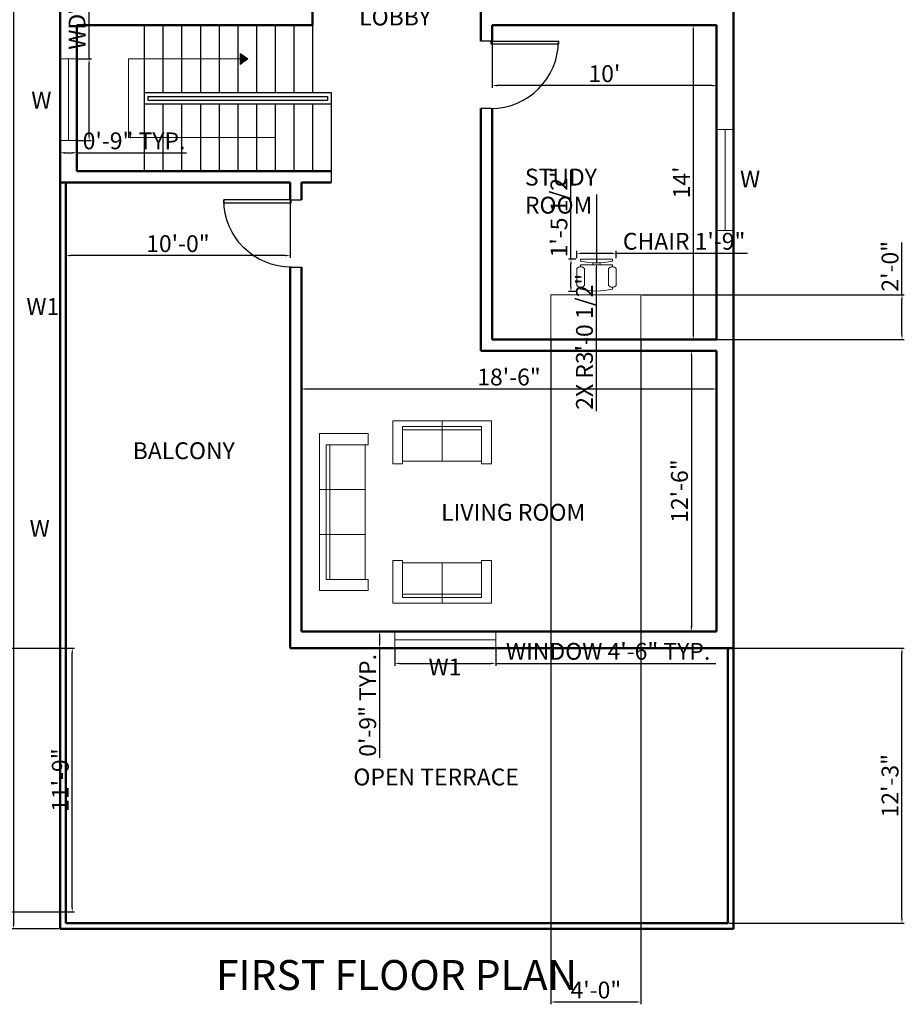
# Model space of a CAD drawing. Units: inches. Extents: x 3587 to 4539, y 1613 to 2440.
# Tile 7 of 8: x 4067 to 4539, y 1613 to 2139. Entities that reach past the tile are written whole.
import ezdxf

# ---------------------------------------------------------------- set-up
doc = ezdxf.new("R2010")
doc.units = ezdxf.units.IN
for name, color, linetype, lineweight in [('A-ANNO-DIMS', 2, 'Continuous', 18), ('A-ANNO-SYMB', 7, 'Continuous', 18), ('A-ANNO-TEXT', 7, 'Continuous', 18), ('A-ANNO-TITL', 7, 'Continuous', 35), ('A-AREA-IDEN', 7, 'Continuous', 25), ('A-DOOR', 3, 'Continuous', 25), ('A-FLOR-STRS', 7, 'Continuous', 25), ('A-FURN', 8, 'Continuous', 18), ('A-GLAZ', 4, 'Continuous', 20), ('A-WALL', 7, 'Continuous', 50)]:
    doc.layers.add(name, color=color, linetype=linetype, lineweight=lineweight)
doc.styles.get("Standard").update_dxf_attribs({"font": 'arial.ttf'})
doc.dimstyles.new('ISO-25', dxfattribs={"dimtxt": 9, "dimasz": 2.5, "dimexe": 1.25, "dimexo": 0.625, "dimtad": 1, "dimlunit": 3, "dimtxsty": 'Standard', "dimcen": 2.5, "dimadec": 0, "dimazin": 0, "dimtfac": 1, "dimtmove": 0, "dimatfit": 3, "dimfxl": 1, "dimarcsym": 0})

# ---------------------------------------------------------------- blocks, each defined once
blk = doc.blocks.new('*U4')
for p, q in [((0, 0), (0, -6)), ((40, 0), (40, -6))]:
    blk.add_line(p, q)
blk.add_lwpolyline([(0, 0), (0, 40), (1.75, 40), (1.75, 0)], close=True)
blk.add_arc((0, 0), 40, 0, 90)
blk = doc.blocks.new('*D28')
at = {"layer": 'A-ANNO-DIMS', "color": 0, "lineweight": -2, "transparency": 16777216}
for p, q in [((4087.49, 2372.93), (4061.98, 2372.93)), ((4063.23, 2370.43), (4063.23, 1655.43)), ((4087.49, 1652.93), (4061.98, 1652.93))]:
    blk.add_line(p, q, dxfattribs=at)
at = {"layer": 'A-ANNO-DIMS', "color": 0, "transparency": 16777216}
for points in [[(4062.81, 2370.43), (4063.65, 2370.43), (4063.23, 2372.93)], [(4062.81, 1655.43), (4063.65, 1655.43), (4063.23, 1652.93)]]:
    blk.add_solid(points, dxfattribs=at)
at = {"layer": 'Defpoints', "color": 0, "transparency": 16777216}
for p in [(4088.12, 2372.93), (4063.23, 1652.93), (4088.12, 1652.93)]:
    blk.add_point(p, dxfattribs=at)
at = {"layer": 'A-ANNO-DIMS', "color": 0, "transparency": 16777216, "insert": (4058.01, 2019.45), "char_height": 9, "attachment_point": 5, "rotation": 90}
blk.add_mtext("60'", dxfattribs=at)
blk = doc.blocks.new('*D37')
at = {"layer": 'A-ANNO-DIMS', "color": 0, "lineweight": -2, "transparency": 16777216}
for p, q in [((4319.12, 2135.31), (4319.12, 2102.45)), ((4439.12, 2135.31), (4439.12, 2102.45)), ((4436.62, 2103.7), (4321.62, 2103.7))]:
    blk.add_line(p, q, dxfattribs=at)
at = {"layer": 'A-ANNO-DIMS', "color": 0, "transparency": 16777216}
for points in [[(4321.62, 2104.12), (4321.62, 2103.28), (4319.12, 2103.7)], [(4436.62, 2104.12), (4436.62, 2103.28), (4439.12, 2103.7)]]:
    blk.add_solid(points, dxfattribs=at)
at = {"layer": 'Defpoints', "color": 0, "transparency": 16777216}
for p in [(4319.12, 2135.93), (4439.12, 2135.93), (4319.12, 2103.7)]:
    blk.add_point(p, dxfattribs=at)
at = {"layer": 'A-ANNO-DIMS', "color": 0, "transparency": 16777216, "insert": (4379.12, 2108.92), "char_height": 9, "attachment_point": 5}
blk.add_mtext("10'", dxfattribs=at)
blk = doc.blocks.new('*D38')
at = {"layer": 'A-ANNO-DIMS', "color": 0, "lineweight": -2, "transparency": 16777216}
for p, q in [((4438.49, 2135.93), (4425.38, 2135.93)), ((4426.63, 2133.43), (4426.63, 1970.43)), ((4438.49, 1967.93), (4425.38, 1967.93))]:
    blk.add_line(p, q, dxfattribs=at)
at = {"layer": 'A-ANNO-DIMS', "color": 0, "transparency": 16777216}
for points in [[(4426.21, 2133.43), (4427.05, 2133.43), (4426.63, 2135.93)], [(4426.21, 1970.43), (4427.05, 1970.43), (4426.63, 1967.93)]]:
    blk.add_solid(points, dxfattribs=at)
at = {"layer": 'Defpoints', "color": 0, "transparency": 16777216}
for p in [(4439.12, 2135.93), (4426.63, 1967.93), (4439.12, 1967.93)]:
    blk.add_point(p, dxfattribs=at)
at = {"layer": 'A-ANNO-DIMS', "color": 0, "transparency": 16777216, "insert": (4421.49, 2051.93), "char_height": 9, "attachment_point": 5, "rotation": 90}
blk.add_mtext("14'", dxfattribs=at)
blk = doc.blocks.new('*D39')
at = {"layer": 'A-ANNO-DIMS', "color": 0, "lineweight": -2, "transparency": 16777216}
for p, q in [((4438.49, 1961.93), (4424.4, 1961.93)), ((4425.65, 1959.43), (4425.65, 1814.43)), ((4438.49, 1811.93), (4424.4, 1811.93))]:
    blk.add_line(p, q, dxfattribs=at)
at = {"layer": 'A-ANNO-DIMS', "color": 0, "transparency": 16777216}
for points in [[(4425.23, 1959.43), (4426.06, 1959.43), (4425.65, 1961.93)], [(4425.23, 1814.43), (4426.06, 1814.43), (4425.65, 1811.93)]]:
    blk.add_solid(points, dxfattribs=at)
at = {"layer": 'Defpoints', "color": 0, "transparency": 16777216}
for p in [(4439.12, 1961.93), (4425.65, 1811.93), (4439.12, 1811.93)]:
    blk.add_point(p, dxfattribs=at)
at = {"layer": 'A-ANNO-DIMS', "color": 0, "transparency": 16777216, "insert": (4420.43, 1886.93), "char_height": 9, "attachment_point": 5, "rotation": 90}
blk.add_mtext('12\'-6"', dxfattribs=at)
blk = doc.blocks.new('Chair - Desk')
for p, q in [((-8.5, 0), (-8.5, -1)), ((-8.5, 0), (8.5, 0)), ((8.5, 0), (8.5, -1)), ((-10.5, -5), (-10.5, -14)), ((-8.5, -3), (-8.5, -4)), ((-8.5, -3), (8.5, -3)), ((-6.5, -14), (-6.5, -5)), ((-2, -3), (-2, -1.9355)), ((2, -1.9576), (2, -3)), ((6.5, -5), (6.5, -14)), ((8.5, -3), (8.5, -4)), ((10.5, -14), (10.5, -5)), ((-8.5, -15), (-8.5, -16)), ((8.5, -15), (8.5, -16))]:
    blk.add_line(p, q)
for centre, radius, start, end in [((-8.5, -6.5), 2.5, 36.8699, 143.1301), ((0, 34.625), 36.625, 256.5803, 283.4197), ((8.5, -6.5), 2.5, 36.8699, 143.1301), ((-8.5, -12.5), 2.5, 216.8699, 323.1301), ((8.5, -12.5), 2.5, 216.8699, 323.1301), ((0, 19.625), 36.625, 256.5803, 283.4197)]:
    blk.add_arc(centre, radius, start, end)
blk = doc.blocks.new('*D42')
at = {"layer": 'A-ANNO-DIMS', "color": 0, "lineweight": -2, "transparency": 16777216}
for p, q in [((4217.12, 1961.31), (4217.12, 1940.26)), ((4439.12, 1961.31), (4439.12, 1940.26)), ((4436.62, 1941.51), (4219.62, 1941.51))]:
    blk.add_line(p, q, dxfattribs=at)
at = {"layer": 'A-ANNO-DIMS', "color": 0, "transparency": 16777216}
for points in [[(4219.62, 1941.93), (4219.62, 1941.1), (4217.12, 1941.51)], [(4436.62, 1941.93), (4436.62, 1941.1), (4439.12, 1941.51)]]:
    blk.add_solid(points, dxfattribs=at)
at = {"layer": 'Defpoints', "color": 0, "transparency": 16777216}
for p in [(4217.12, 1961.93), (4439.12, 1961.93), (4217.12, 1941.51)]:
    blk.add_point(p, dxfattribs=at)
at = {"layer": 'A-ANNO-DIMS', "color": 0, "transparency": 16777216, "insert": (4328.12, 1946.73), "char_height": 9, "attachment_point": 5}
blk.add_mtext('18\'-6"', dxfattribs=at)
blk = doc.blocks.new('STAIR-DOGLEG')
for p, q in [((0, 84), (0, 6)), ((10, 84), (10, 48)), ((20, 84), (20, 48)), ((30, 84), (30, 48)), ((40, 84), (40, 48)), ((50, 84), (50, 48)), ((60, 84), (60, 48)), ((70, 84), (70, 48)), ((80, 84), (80, 48)), ((90, 84), (90, 48)), ((0, 48), (100, 48)), ((100, 48), (100, 0)), ((2, 46), (98, 46)), ((2, 46), (2, 44)), ((2, 44), (98, 44)), ((98, 46), (98, 44)), ((0, 42), (100, 42)), ((10, 42), (10, 6)), ((20, 42), (20, 6)), ((30, 42), (30, 6)), ((40, 42), (40, 6)), ((50, 42), (50, 6)), ((60, 42), (60, 6)), ((70, 42), (70, 6)), ((80, 42), (80, 6)), ((90, 42), (90, 6))]:
    blk.add_line(p, q)
blk = doc.blocks.new('STAIR-PATH-ARROW')
h = blk.add_hatch(color=256)
h.dxf.hatch_style = 1
h.paths.add_polyline_path([(63.77, 42), (59.72, 42), (59.72, 39.06)])
h.paths.add_polyline_path([(59.72, 44.94), (59.72, 42), (63.77, 42)])
for p, q in [((63.77, 42), (59.72, 44.94)), ((59.72, 44.94), (59.72, 42)), ((0, 0), (0, 42)), ((0, 42), (63.77, 42)), ((63.77, 42), (59.72, 39.06)), ((59.72, 39.06), (59.72, 42)), ((78.41, 0), (0, 0))]:
    blk.add_line(p, q)
blk = doc.blocks.new('SOFA-3-SEAT-84IN')
for p, q in [((0, 0), (0, 84)), ((26, 78), (3.47, 78)), ((3.47, 78), (3.47, 6)), ((5.38, 6), (5.38, 78)), ((24.44, 6), (24.44, 78)), ((24.44, 54), (0, 54)), ((24.44, 30), (0, 30)), ((26, 6), (3.47, 6))]:
    blk.add_line(p, q)
for points in [[(0, 84), (26, 84), (26, 78)], [(26, 6), (26, 0), (0, 0)]]:
    blk.add_lwpolyline(points)
blk = doc.blocks.new('LOVESEAT-2-SEAT')
for p, q in [((5.28, 22.88), (5.28, 3.05)), ((5.28, 21.51), (47.52, 21.51)), ((26.4, 21.51), (26.4, 0)), ((47.52, 22.88), (47.52, 3.05)), ((0, 0), (52.8, 0)), ((5.28, 4.74), (47.52, 4.74)), ((47.52, 3.05), (5.28, 3.05))]:
    blk.add_line(p, q)
for points in [[(5.28, 22.88), (0, 22.88), (0, 0)], [(52.8, 0), (52.8, 22.88), (47.52, 22.88)]]:
    blk.add_lwpolyline(points)
blk = doc.blocks.new('WINDOW-54IN')
for p, q in [((9, 54), (0, 54)), ((4.5, 54), (4.5, 0)), ((9, 0), (0, 0))]:
    blk.add_line(p, q)
blk = doc.blocks.new('WINDOW-43_61IN')
for p, q in [((9, 43.61), (0, 43.61)), ((4.5, 0), (4.5, 43.61)), ((9, 0), (0, 0))]:
    blk.add_line(p, q)
blk = doc.blocks.new('*D54')
at = {"layer": 'A-ANNO-DIMS', "color": 0, "lineweight": -2, "transparency": 16777216}
for p, q in [((4267.04, 1802.31), (4267.04, 1793.58)), ((4321.04, 1802.31), (4321.04, 1793.58)), ((4269.54, 1794.83), (4318.54, 1794.83)), ((4321.04, 1794.83), (4438.68, 1794.83))]:
    blk.add_line(p, q, dxfattribs=at)
at = {"layer": 'A-ANNO-DIMS', "color": 0, "transparency": 16777216}
for points in [[(4269.54, 1795.25), (4269.54, 1794.42), (4267.04, 1794.83)], [(4318.54, 1795.25), (4318.54, 1794.42), (4321.04, 1794.83)]]:
    blk.add_solid(points, dxfattribs=at)
at = {"layer": 'Defpoints', "color": 0, "transparency": 16777216}
for p in [(4267.04, 1802.93), (4321.04, 1802.93), (4321.04, 1794.83)]:
    blk.add_point(p, dxfattribs=at)
at = {"layer": 'A-ANNO-DIMS', "color": 0, "transparency": 16777216, "insert": (4381.11, 1800.11), "char_height": 9, "attachment_point": 5}
blk.add_mtext('WINDOW 4\'-6" TYP.', dxfattribs=at)
blk = doc.blocks.new('*D55')
at = {"layer": 'A-ANNO-DIMS', "color": 0, "lineweight": -2, "transparency": 16777216}
for p, q in [((4266.42, 1811.93), (4257.69, 1811.93)), ((4258.94, 1809.43), (4258.94, 1805.43)), ((4266.42, 1802.93), (4257.69, 1802.93)), ((4258.94, 1802.93), (4258.94, 1744.32))]:
    blk.add_line(p, q, dxfattribs=at)
at = {"layer": 'A-ANNO-DIMS', "color": 0, "transparency": 16777216}
for points in [[(4258.53, 1809.43), (4259.36, 1809.43), (4258.94, 1811.93)], [(4258.53, 1805.43), (4259.36, 1805.43), (4258.94, 1802.93)]]:
    blk.add_solid(points, dxfattribs=at)
at = {"layer": 'Defpoints', "color": 0, "transparency": 16777216}
for p in [(4267.04, 1811.93), (4258.94, 1802.93), (4267.04, 1802.93)]:
    blk.add_point(p, dxfattribs=at)
at = {"layer": 'A-ANNO-DIMS', "color": 0, "transparency": 16777216, "insert": (4253.72, 1772.38), "char_height": 9, "attachment_point": 5, "rotation": 90}
blk.add_mtext('0\'-9" TYP.', dxfattribs=at)
blk = doc.blocks.new('*D58')
at = {"layer": 'A-ANNO-DIMS', "color": 0, "lineweight": -2, "transparency": 16777216}
for p, q in [((4103.66, 2117.93), (4103.66, 2234.19)), ((4097.74, 2117.93), (4104.91, 2117.93)), ((4103.66, 2076.82), (4103.66, 2115.43)), ((4097.74, 2074.32), (4104.91, 2074.32))]:
    blk.add_line(p, q, dxfattribs=at)
at = {"layer": 'A-ANNO-DIMS', "color": 0, "transparency": 16777216}
for points in [[(4103.24, 2115.43), (4104.07, 2115.43), (4103.66, 2117.93)], [(4103.24, 2076.82), (4104.07, 2076.82), (4103.66, 2074.32)]]:
    blk.add_solid(points, dxfattribs=at)
at = {"layer": 'Defpoints', "color": 0, "transparency": 16777216}
for p in [(4097.12, 2117.93), (4103.66, 2117.93), (4097.12, 2074.32)]:
    blk.add_point(p, dxfattribs=at)
at = {"layer": 'A-ANNO-DIMS', "color": 0, "transparency": 16777216, "insert": (4098.38, 2177.31), "char_height": 9, "attachment_point": 5, "rotation": 90}
blk.add_mtext('WDW 3\'-7 1/2" TYP.', dxfattribs=at)
blk = doc.blocks.new('*D59')
at = {"layer": 'A-ANNO-DIMS', "color": 0, "lineweight": -2, "transparency": 16777216}
for p, q in [((4088.12, 2073.7), (4088.12, 2066.53)), ((4097.12, 2073.7), (4097.12, 2066.53)), ((4090.62, 2067.78), (4094.62, 2067.78)), ((4097.12, 2067.78), (4155.73, 2067.78))]:
    blk.add_line(p, q, dxfattribs=at)
at = {"layer": 'A-ANNO-DIMS', "color": 0, "transparency": 16777216}
for points in [[(4090.62, 2068.2), (4090.62, 2067.37), (4088.12, 2067.78)], [(4094.62, 2068.2), (4094.62, 2067.37), (4097.12, 2067.78)]]:
    blk.add_solid(points, dxfattribs=at)
at = {"layer": 'Defpoints', "color": 0, "transparency": 16777216}
for p in [(4088.12, 2074.32), (4097.12, 2074.32), (4097.12, 2067.78)]:
    blk.add_point(p, dxfattribs=at)
at = {"layer": 'A-ANNO-DIMS', "color": 0, "transparency": 16777216, "insert": (4127.67, 2073), "char_height": 9, "attachment_point": 5}
blk.add_mtext('0\'-9" TYP.', dxfattribs=at)
blk = doc.blocks.new('*D68')
at = {"layer": 'A-ANNO-DIMS', "color": 0, "lineweight": -2, "transparency": 16777216}
for p, q in [((4364.4, 2011.51), (4364.4, 2015.29)), ((4366.9, 2014.04), (4382.9, 2014.04)), ((4385.4, 2011.51), (4385.4, 2015.29)), ((4385.4, 2014.04), (4455.59, 2014.04))]:
    blk.add_line(p, q, dxfattribs=at)
at = {"layer": 'A-ANNO-DIMS', "color": 0, "transparency": 16777216}
for points in [[(4366.9, 2014.45), (4366.9, 2013.62), (4364.4, 2014.04)], [(4382.9, 2014.45), (4382.9, 2013.62), (4385.4, 2014.04)]]:
    blk.add_solid(points, dxfattribs=at)
at = {"layer": 'Defpoints', "color": 0, "transparency": 16777216}
for p in [(4364.4, 2010.89), (4385.4, 2014.04), (4385.4, 2010.89)]:
    blk.add_point(p, dxfattribs=at)
at = {"layer": 'A-ANNO-DIMS', "color": 0, "transparency": 16777216, "insert": (4421.75, 2019.31), "char_height": 9, "attachment_point": 5}
blk.add_mtext('CHAIR 1\'-9"', dxfattribs=at)
blk = doc.blocks.new('*D69')
at = {"layer": 'A-ANNO-DIMS', "color": 0, "lineweight": -2, "transparency": 16777216}
for p, q in [((4361.25, 2010.89), (4361.25, 2058.68)), ((4363.78, 2010.89), (4360, 2010.89)), ((4361.25, 1996.05), (4361.25, 2008.39)), ((4363.78, 1993.55), (4360, 1993.55))]:
    blk.add_line(p, q, dxfattribs=at)
at = {"layer": 'A-ANNO-DIMS', "color": 0, "transparency": 16777216}
for points in [[(4360.84, 2008.39), (4361.67, 2008.39), (4361.25, 2010.89)], [(4360.84, 1996.05), (4361.67, 1996.05), (4361.25, 1993.55)]]:
    blk.add_solid(points, dxfattribs=at)
at = {"layer": 'Defpoints', "color": 0, "transparency": 16777216}
for p in [(4361.25, 2010.89), (4364.4, 2010.89), (4364.4, 1993.55)]:
    blk.add_point(p, dxfattribs=at)
at = {"layer": 'A-ANNO-DIMS', "color": 0, "transparency": 16777216, "insert": (4355.98, 2036.03), "char_height": 9, "attachment_point": 5, "rotation": 90}
blk.add_mtext('1\'-5 1/2"', dxfattribs=at)
blk = doc.blocks.new('*D80')
at = {"layer": 'A-ANNO-DIMS', "color": 0, "lineweight": -2, "transparency": 16777216}
for p, q in [((3996.15, 1802.93), (4095.87, 1802.93)), ((4094.62, 1664.43), (4094.62, 1800.43)), ((3996.15, 1661.93), (4095.87, 1661.93))]:
    blk.add_line(p, q, dxfattribs=at)
at = {"layer": 'A-ANNO-DIMS', "color": 0, "transparency": 16777216}
for points in [[(4094.21, 1800.43), (4095.04, 1800.43), (4094.62, 1802.93)], [(4094.21, 1664.43), (4095.04, 1664.43), (4094.62, 1661.93)]]:
    blk.add_solid(points, dxfattribs=at)
at = {"layer": 'Defpoints', "color": 0, "transparency": 16777216}
for p in [(3995.52, 1802.93), (4094.62, 1802.93), (3995.52, 1661.93)]:
    blk.add_point(p, dxfattribs=at)
at = {"layer": 'A-ANNO-DIMS', "color": 0, "transparency": 16777216, "insert": (4089.4, 1732.43), "char_height": 9, "attachment_point": 5, "rotation": 90}
blk.add_mtext('11\'-9"', dxfattribs=at)
blk = doc.blocks.new('*D81')
at = {"layer": 'A-ANNO-DIMS', "color": 0, "lineweight": -2, "transparency": 16777216}
for p, q in [((4091.12, 2051.31), (4091.12, 2011.58)), ((4211.12, 2051.31), (4211.12, 2011.58)), ((4208.62, 2012.83), (4093.62, 2012.83))]:
    blk.add_line(p, q, dxfattribs=at)
at = {"layer": 'A-ANNO-DIMS', "color": 0, "transparency": 16777216}
for points in [[(4093.62, 2013.25), (4093.62, 2012.42), (4091.12, 2012.83)], [(4208.62, 2013.25), (4208.62, 2012.42), (4211.12, 2012.83)]]:
    blk.add_solid(points, dxfattribs=at)
at = {"layer": 'Defpoints', "color": 0, "transparency": 16777216}
for p in [(4091.12, 2051.93), (4211.12, 2051.93), (4091.12, 2012.83)]:
    blk.add_point(p, dxfattribs=at)
at = {"layer": 'A-ANNO-DIMS', "color": 0, "transparency": 16777216, "insert": (4151.12, 2018.05), "char_height": 9, "attachment_point": 5}
blk.add_mtext('10\'-0"', dxfattribs=at)
blk = doc.blocks.new('*D82')
at = {"layer": 'A-ANNO-DIMS', "color": 0, "lineweight": -2, "transparency": 16777216}
for p, q in [((4445.74, 1802.93), (4539.47, 1802.93)), ((4538.22, 1658.43), (4538.22, 1800.43)), ((4445.74, 1655.93), (4539.47, 1655.93))]:
    blk.add_line(p, q, dxfattribs=at)
at = {"layer": 'A-ANNO-DIMS', "color": 0, "transparency": 16777216}
for points in [[(4537.8, 1800.43), (4538.63, 1800.43), (4538.22, 1802.93)], [(4537.8, 1658.43), (4538.63, 1658.43), (4538.22, 1655.93)]]:
    blk.add_solid(points, dxfattribs=at)
at = {"layer": 'Defpoints', "color": 0, "transparency": 16777216}
for p in [(4445.12, 1802.93), (4538.22, 1802.93), (4445.12, 1655.93)]:
    blk.add_point(p, dxfattribs=at)
at = {"layer": 'A-ANNO-DIMS', "color": 0, "transparency": 16777216, "insert": (4532.99, 1729.43), "char_height": 9, "attachment_point": 5, "rotation": 90}
blk.add_mtext('12\'-3"', dxfattribs=at)
blk = doc.blocks.new('*D86')
at = {"layer": 'A-ANNO-DIMS', "color": 0, "lineweight": -2, "transparency": 16777216}
for p, q in [((4350.57, 1967.31), (4350.57, 1612.58)), ((4398.57, 1967.31), (4398.57, 1612.58)), ((4353.07, 1613.83), (4396.07, 1613.83))]:
    blk.add_line(p, q, dxfattribs=at)
at = {"layer": 'A-ANNO-DIMS', "color": 0, "transparency": 16777216}
for points in [[(4353.07, 1614.25), (4353.07, 1613.42), (4350.57, 1613.83)], [(4396.07, 1614.25), (4396.07, 1613.42), (4398.57, 1613.83)]]:
    blk.add_solid(points, dxfattribs=at)
at = {"layer": 'Defpoints', "color": 0, "transparency": 16777216}
for p in [(4350.57, 1967.93), (4398.57, 1967.93), (4398.57, 1613.83)]:
    blk.add_point(p, dxfattribs=at)
at = {"layer": 'A-ANNO-DIMS', "color": 0, "transparency": 16777216, "insert": (4374.57, 1619.05), "char_height": 9, "attachment_point": 5}
blk.add_mtext('4\'-0"', dxfattribs=at)
blk = doc.blocks.new('*D87')
at = {"layer": 'A-ANNO-DIMS', "color": 0, "lineweight": -2, "transparency": 16777216}
for p, q in [((4538.22, 1991.93), (4538.22, 2019.76)), ((4399.19, 1991.93), (4539.47, 1991.93)), ((4538.22, 1970.43), (4538.22, 1989.43)), ((4399.19, 1967.93), (4539.47, 1967.93))]:
    blk.add_line(p, q, dxfattribs=at)
at = {"layer": 'A-ANNO-DIMS', "color": 0, "transparency": 16777216}
for points in [[(4537.8, 1989.43), (4538.63, 1989.43), (4538.22, 1991.93)], [(4537.8, 1970.43), (4538.63, 1970.43), (4538.22, 1967.93)]]:
    blk.add_solid(points, dxfattribs=at)
at = {"layer": 'Defpoints', "color": 0, "transparency": 16777216}
for p in [(4398.57, 1991.93), (4538.22, 1991.93), (4398.57, 1967.93)]:
    blk.add_point(p, dxfattribs=at)
at = {"layer": 'A-ANNO-DIMS', "color": 0, "transparency": 16777216, "insert": (4533, 2007.1), "char_height": 9, "attachment_point": 5, "rotation": 90}
blk.add_mtext('2\'-0"', dxfattribs=at)
blk = doc.blocks.new('*D100')
at = {"layer": 'A-ANNO-DIMS', "color": 0, "lineweight": -2, "transparency": 16777216}
for p, q in [((4374.9, 2045.51), (4374.9, 2008.89)), ((4374.9, 1929.63), (4374.9, 2006.39))]:
    blk.add_line(p, q, dxfattribs=at)
at = {"layer": 'A-ANNO-DIMS', "color": 0, "transparency": 16777216}
blk.add_solid([(4374.49, 2006.39), (4375.32, 2006.39), (4374.9, 2008.89)], dxfattribs=at)
at = {"layer": 'Defpoints', "color": 0, "transparency": 16777216}
for p in [(4374.9, 2045.51), (4374.9, 2008.89)]:
    blk.add_point(p, dxfattribs=at)
at = {"layer": 'A-ANNO-DIMS', "color": 0, "transparency": 16777216, "insert": (4369.62, 1966.76), "char_height": 9, "attachment_point": 5, "rotation": 89.9993}
blk.add_mtext('2X R3\'-0 1/2"', dxfattribs=at)

msp = doc.modelspace()

# ---------------------------------------------------------------- linework, layer by layer
at = {"layer": 'A-FURN'}
for p, q in [((4350.566, 1967.933), (4350.566, 1991.933)), ((4350.566, 1991.933), (4398.566, 1991.933)), ((4398.566, 1991.933), (4398.566, 1967.933))]:
    msp.add_line(p, q, dxfattribs=at)
at = {"layer": 'A-WALL'}
for p, q in [((4088.116, 2372.933), (4088.116, 1652.933)), ((4448.116, 2372.933), (4448.116, 1652.933)), ((4223.116, 2213.933), (4223.116, 2135.933)), ((4313.116, 2213.933), (4313.116, 2135.933)), ((4223.116, 2135.933), (4097.116, 2135.933)), ((4097.116, 2135.933), (4097.116, 2057.933)), ((4313.116, 2135.933), (4313.116, 2127.481)), ((4439.116, 2135.933), (4319.116, 2135.933)), ((4319.116, 2135.933), (4319.116, 2127.481)), ((4439.116, 2135.933), (4439.116, 1967.933)), ((4313.116, 2091.481), (4313.116, 1961.933)), ((4319.116, 2091.486), (4319.116, 1967.933)), ((4233.116, 2057.933), (4097.116, 2057.933)), ((4211.116, 2051.933), (4088.116, 2051.933)), ((4091.116, 2051.933), (4091.116, 1655.933)), ((4211.116, 2051.933), (4211.116, 2042.577)), ((4233.116, 2051.933), (4217.116, 2051.933)), ((4217.116, 2051.933), (4217.116, 2042.577)), ((4211.116, 2006.582), (4211.116, 1925.933)), ((4217.116, 2006.577), (4217.116, 1811.933)), ((4439.116, 1967.933), (4319.116, 1967.933)), ((4439.116, 1961.933), (4313.116, 1961.933)), ((4439.116, 1961.933), (4439.116, 1811.933)), ((4211.116, 1925.933), (4211.116, 1802.933)), ((4439.116, 1811.933), (4217.116, 1811.933)), ((4448.116, 1802.933), (4211.116, 1802.933)), ((4445.116, 1802.933), (4445.116, 1655.933)), ((4088.116, 1654.933), (4088.116, 1652.933)), ((4448.116, 1652.933), (4088.116, 1652.933)), ((4445.116, 1655.933), (4091.116, 1655.933)), ((4448.116, 1654.933), (4448.116, 1652.933))]:
    msp.add_line(p, q, dxfattribs=at)

# ---------------------------------------------------------------- block references
at = {"layer": 'A-ANNO-SYMB'}
msp.add_blockref('STAIR-PATH-ARROW', (4124.703, 2075.933), dxfattribs=at)
at = {"layer": 'A-DOOR', "yscale": 0.9, "zscale": 0.9}
for p, xscale, rotation in [((4318.516, 2127.481), 0.9, 270), ((4211.716, 2042.577), -0.9, 90)]:
    msp.add_blockref('*U4', p, dxfattribs=dict(at, xscale=xscale, rotation=rotation))
at = {"layer": 'A-FLOR-STRS'}
msp.add_blockref('STAIR-DOGLEG', (4133.115, 2051.933), dxfattribs=at)
at = {"layer": 'A-FURN'}
for name, p in [('Chair - Desk', (4374.904, 2010.885)), ('SOFA-3-SEAT-84IN', (4226.869, 1833.732)), ('LOVESEAT-2-SEAT', (4265.933, 1827.017))]:
    msp.add_blockref(name, p, dxfattribs=at)
at = {"layer": 'A-FURN', "extrusion": (0, 0, -1), "zscale": -1, "rotation": 180}
msp.add_blockref('LOVESEAT-2-SEAT', (-4265.933, 1924.448), dxfattribs=at)
at = {"layer": 'A-GLAZ'}
for name, p in [('WINDOW-43_61IN', (4088.115, 2074.325)), ('WINDOW-54IN', (4439.115, 2026.316))]:
    msp.add_blockref(name, p, dxfattribs=at)
at = {"layer": 'A-GLAZ', "rotation": 270}
msp.add_blockref('WINDOW-54IN', (4267.045, 1811.933), dxfattribs=at)

# ---------------------------------------------------------------- texts
at = {"layer": 'A-ANNO-TEXT', "char_height": 9, "attachment_point": 1}
for s, width, insert in [('W', 47.85632, (4072.738, 2100.404)), ('W', 47.85632, (4451.629, 2058.251)), ('W1', 34.45655, (4070.091, 1990.101)), ('W', 47.85632, (4071.826, 1871.518)), ('W1', 34.45655, (4285.084, 1797.437))]:
    msp.add_mtext_dynamic_manual_height_columns(s, width=width, gutter_width=12.5, heights=[0], dxfattribs=dict(at, insert=insert))
at = {"layer": 'A-ANNO-TITL', "insert": (4171.493, 1636.232), "char_height": 16, "attachment_point": 1}
msp.add_mtext_dynamic_manual_height_columns('FIRST FLOOR PLAN', width=347.53883, gutter_width=12.5, heights=[0], dxfattribs=at)
at = {"layer": 'A-AREA-IDEN', "char_height": 9, "attachment_point": 1}
for s, width, insert in [('LOBBY', 107.19817, (4248.017, 2144.864)), ('STUDY \\PROOM', 136.86909, (4336.628, 2059.283)), ('BALCONY', 107.19817, (4126.972, 1913.009)), ('LIVING ROOM ', 173.2399, (4291.844, 1880.1)), ('OPEN TERRACE', 107.19817, (4244.93, 1738.593))]:
    msp.add_mtext_dynamic_manual_height_columns(s, width=width, gutter_width=12.5, heights=[0], dxfattribs=dict(at, insert=insert))

# ---------------------------------------------------------------- dimensions: what is measured, and where the dimension line sits
at = {"layer": 'A-ANNO-DIMS'}
dim = msp.add_linear_dim(base=(4063.23, 1652.933), p1=(4088.116, 2372.933), p2=(4088.116, 1652.933), angle=90, dimstyle='ISO-25', override={"dimclrd": 0, "dimclre": 0, "dimclrt": 0}, dxfattribs=at)
dim.commit()
dim.dimension.update_dxf_attribs({"geometry": '*D28', "text_midpoint": (4063.23, 2019.453), "dimtype": 160})
for base, p1, p2, angle, text, picture, middle in [((4103.657, 2117.933), (4097.116, 2074.325), (4097.116, 2117.933), 90, 'WDW <> TYP.', '*D58', (4098.375, 2177.311)), ((4258.944, 1802.933), (4267.044, 1811.933), (4267.044, 1802.933), 270, '<> TYP.', '*D55', (4253.724, 1772.378))]:
    dim = msp.add_linear_dim(base=base, p1=p1, p2=p2, angle=angle, text=text, dimstyle='ISO-25', override={"dimdec": 1, "dimlfac": 1, "dimrnd": 0, "dimzin": 1, "dimdsep": 46, "dimlunit": 4, "dimfrac": 2}, dxfattribs=at)
    dim.commit()
    dim.dimension.update_dxf_attribs({"geometry": picture, "text_midpoint": middle})
for base, p1, p2, override, picture, middle in [((4319.116, 2103.698), (4439.116, 2135.933), (4319.116, 2135.933), {"dimclrd": 0, "dimclre": 0, "dimclrt": 0}, '*D37', (4379.116, 2108.919)), ((4398.566, 1613.833), (4350.566, 1967.933), (4398.566, 1967.933), {"dimdec": 1, "dimlfac": 1, "dimrnd": 0, "dimzin": 1, "dimdsep": 46, "dimlunit": 4, "dimfrac": 2}, '*D86', (4374.566, 1619.053)), ((4217.116, 1941.513), (4439.116, 1961.933), (4217.116, 1961.933), {"dimclrd": 0, "dimclre": 0, "dimclrt": 0}, '*D42', (4328.116, 1946.733))]:
    dim = msp.add_linear_dim(base=base, p1=p1, p2=p2, dimstyle='ISO-25', override=override, dxfattribs=at)
    dim.commit()
    dim.dimension.update_dxf_attribs({"geometry": picture, "text_midpoint": middle})
for base, p1, p2, angle, override, picture, middle in [((4426.631, 1967.933), (4439.116, 2135.933), (4439.116, 1967.933), 90, {"dimclrd": 0, "dimclre": 0, "dimclrt": 0}, '*D38', (4421.488, 2051.933)), ((4361.254, 2010.885), (4364.404, 1993.552), (4364.404, 2010.885), 90, {"dimdec": 1, "dimlfac": 1, "dimrnd": 0, "dimzin": 1, "dimdsep": 46, "dimlunit": 4, "dimfrac": 2}, '*D69', (4355.976, 2036.034)), ((4091.116, 2012.833), (4211.116, 2051.933), (4091.116, 2051.933), 180, {"dimdec": 1, "dimlfac": 1, "dimrnd": 0, "dimzin": 1, "dimdsep": 46, "dimlunit": 4, "dimfrac": 2}, '*D81', (4151.116, 2018.053)), ((4538.216, 1991.933), (4398.566, 1967.933), (4398.566, 1991.933), 90, {"dimdec": 1, "dimlfac": 1, "dimrnd": 0, "dimzin": 1, "dimdsep": 46, "dimlunit": 4, "dimfrac": 2}, '*D87', (4532.995, 2007.097)), ((4425.647, 1811.933), (4439.116, 1961.933), (4439.116, 1811.933), 90, {"dimclrd": 0, "dimclre": 0, "dimclrt": 0}, '*D39', (4420.427, 1886.933)), ((4094.623, 1802.933), (3995.523, 1661.933), (3995.523, 1802.933), 90, {"dimdec": 1, "dimlfac": 1, "dimrnd": 0, "dimzin": 1, "dimdsep": 46, "dimlunit": 4, "dimfrac": 2}, '*D80', (4089.403, 1732.433)), ((4538.216, 1802.933), (4445.116, 1655.933), (4445.116, 1802.933), 90, {"dimdec": 1, "dimlfac": 1, "dimrnd": 0, "dimzin": 1, "dimdsep": 46, "dimlunit": 4, "dimfrac": 2}, '*D82', (4532.992, 1729.433))]:
    dim = msp.add_linear_dim(base=base, p1=p1, p2=p2, angle=angle, dimstyle='ISO-25', override=override, dxfattribs=at)
    dim.commit()
    dim.dimension.update_dxf_attribs({"geometry": picture, "text_midpoint": middle})
for base, p1, p2, text, picture, middle in [((4097.116, 2067.783), (4088.116, 2074.325), (4097.116, 2074.325), '<> TYP.', '*D59', (4127.67, 2073.003)), ((4385.404, 2014.035), (4364.404, 2010.885), (4385.404, 2010.885), 'CHAIR <>', '*D68', (4421.745, 2019.314)), ((4321.044, 1794.833), (4267.044, 1802.933), (4321.044, 1802.933), 'WINDOW <> TYP.', '*D54', (4381.113, 1800.115))]:
    dim = msp.add_linear_dim(base=base, p1=p1, p2=p2, text=text, dimstyle='ISO-25', override={"dimdec": 1, "dimlfac": 1, "dimrnd": 0, "dimzin": 1, "dimdsep": 46, "dimlunit": 4, "dimfrac": 2}, dxfattribs=at)
    dim.commit()
    dim.dimension.update_dxf_attribs({"geometry": picture, "text_midpoint": middle})
dim = msp.add_radius_dim(center=(4374.904, 2045.51), mpoint=(4374.904, 2008.885), text='2X <>', dimstyle='ISO-25', override={"dimdec": 1, "dimlfac": 1, "dimrnd": 0, "dimzin": 1, "dimdsep": 46, "dimlunit": 4, "dimfrac": 2}, dxfattribs=at)
dim.commit()
dim.dimension.update_dxf_attribs({"geometry": '*D100', "text_midpoint": (4369.622, 1966.76)})

doc.saveas('drawing.dxf')
